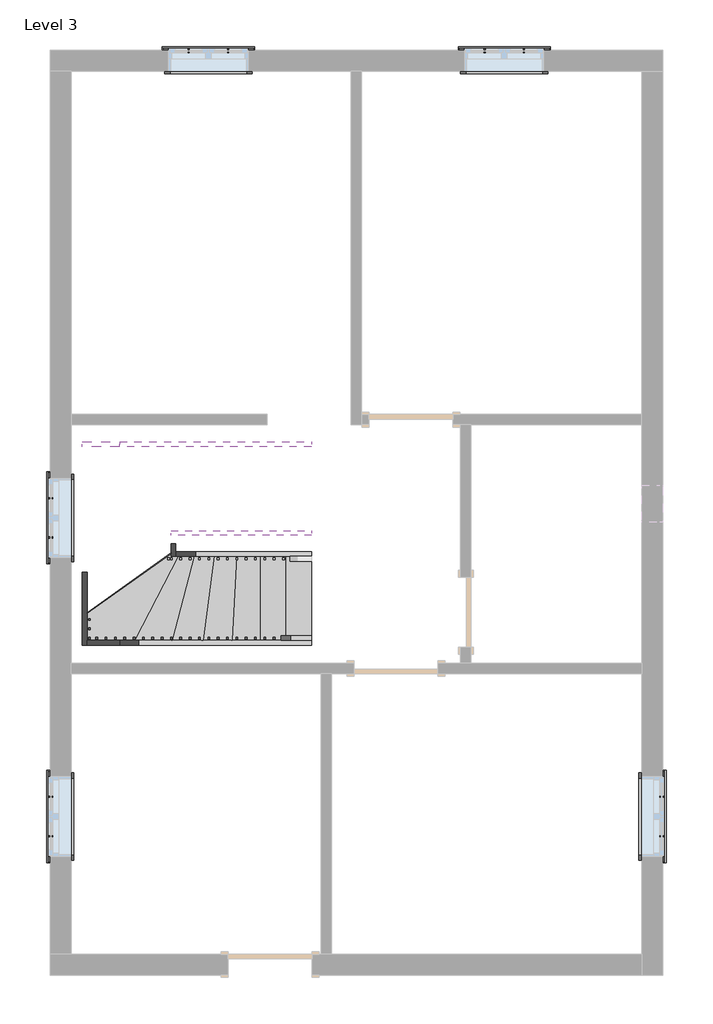
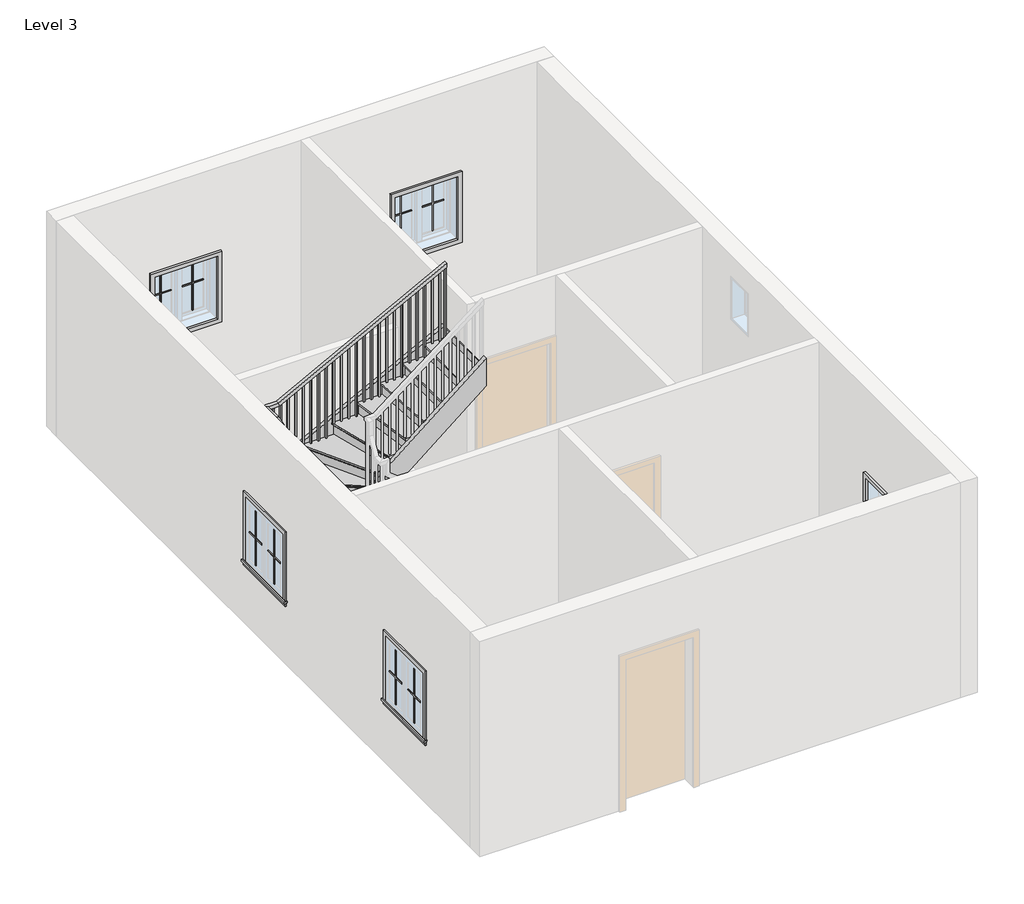
# One storey, part 2 of 2: 20 proxies, 8 members, 1 railing, 1 stair flight.
"""IFC4 building model written with IfcOpenShell, lengths in millimetres."""

from ifc_helpers import new_model, si_unit, frame, origin, place, context, project, spatial, polyline, outline, extrude, faceted_brep, transform, mapped, element, save
from components import muntin_pattern_2x2_muntin_pattern_2x2_b3fe6957, muntin_pattern_2x2_muntin_pattern_2x2_3e0ecaf2, trim_window_exterior_flat_with_sill_41619996, trim_window_interior_flat_picture_frame_51c85655, stair_flight_5420025d

model = new_model("IFC4")

# Units and contexts
model_context = context("Model", 3, world=origin())
ifc_project = project(units=[si_unit("LENGTHUNIT", "METRE", prefix="MILLI")], contexts=[model_context])

# Site, building, storey
site = spatial("IfcSite", under=ifc_project)
building = spatial("IfcBuilding", under=site)
storey = spatial("IfcBuildingStorey", under=building, Name="Level 3", Elevation=3200.4)

# Proxies
placement = place(None, origin())
muntin_pattern_2x2_muntin_pattern_2x2_shape = muntin_pattern_2x2_muntin_pattern_2x2_b3fe6957(model_context)
element("IfcBuildingElementProxy", 1, Name="Muntin Pattern_2x2 : Muntin Pattern_2x2", ObjectType="Muntin Pattern_2x2 : Muntin Pattern_2x2", at=placement, inside=storey, context=model_context, shape_type="MappedRepresentation", body=[
    mapped(muntin_pattern_2x2_muntin_pattern_2x2_shape, transform((-3096.8324167, 5150.2179147, 4184.65), x_axis=(1.0, 0.0, 0.0), y_axis=(0.0, 1.0, 0.0), z_axis=(0.0, 0.0, 1.0))),
])
element("IfcBuildingElementProxy", 2, Name="Muntin Pattern_2x2 : Muntin Pattern_2x2", ObjectType="Muntin Pattern_2x2 : Muntin Pattern_2x2", at=placement, inside=storey, context=model_context, shape_type="MappedRepresentation", body=[
    mapped(muntin_pattern_2x2_muntin_pattern_2x2_shape, transform((122.6175833, 5150.2179147, 4184.65), x_axis=(1.0, 0.0, 0.0), y_axis=(0.0, 1.0, 0.0), z_axis=(0.0, 0.0, 1.0))),
])
element("IfcBuildingElementProxy", 3, Name="Muntin Pattern_2x2 : Muntin Pattern_2x2", ObjectType="Muntin Pattern_2x2 : Muntin Pattern_2x2", at=placement, inside=storey, context=model_context, shape_type="MappedRepresentation", body=[
    mapped(muntin_pattern_2x2_muntin_pattern_2x2_shape, transform((-4597.0199167, -3388.9445853, 4184.65), x_axis=(0.0, 1.0, 0.0), y_axis=(-1.0, 0.0, 0.0), z_axis=(0.0, 0.0, 1.0))),
])
element("IfcBuildingElementProxy", 4, Name="Muntin Pattern_2x2 : Muntin Pattern_2x2", ObjectType="Muntin Pattern_2x2 : Muntin Pattern_2x2", at=placement, inside=storey, context=model_context, shape_type="MappedRepresentation", body=[
    mapped(muntin_pattern_2x2_muntin_pattern_2x2_shape, transform((2051.4300833, -2960.3195853, 4184.65), x_axis=(0.0, -1.0, 0.0), y_axis=(1.0, 0.0, 0.0), z_axis=(0.0, 0.0, 1.0))),
])
element("IfcBuildingElementProxy", 5, Name="Muntin Pattern_2x2 : Muntin Pattern_2x2", ObjectType="Muntin Pattern_2x2 : Muntin Pattern_2x2", at=placement, inside=storey, context=model_context, shape_type="MappedRepresentation", body=[
    mapped(muntin_pattern_2x2_muntin_pattern_2x2_shape, transform((-4597.0199167, -140.9195853, 4184.65), x_axis=(0.0, 1.0, 0.0), y_axis=(-1.0, 0.0, 0.0), z_axis=(0.0, 0.0, 1.0))),
])
muntin_pattern_2x2_muntin_pattern_2x2_2_shape = muntin_pattern_2x2_muntin_pattern_2x2_3e0ecaf2(model_context)
element("IfcBuildingElementProxy", 6, Name="Muntin Pattern_2x2 : Muntin Pattern_2x2", ObjectType="Muntin Pattern_2x2 : Muntin Pattern_2x2", at=placement, inside=storey, context=model_context, shape_type="MappedRepresentation", body=[
    mapped(muntin_pattern_2x2_muntin_pattern_2x2_2_shape, transform((-2668.2074167, 5150.2179147, 4184.65), x_axis=(-1.0, 0.0, 0.0), y_axis=(0.0, -1.0, 0.0), z_axis=(0.0, 0.0, 1.0))),
])
element("IfcBuildingElementProxy", 7, Name="Muntin Pattern_2x2 : Muntin Pattern_2x2", ObjectType="Muntin Pattern_2x2 : Muntin Pattern_2x2", at=placement, inside=storey, context=model_context, shape_type="MappedRepresentation", body=[
    mapped(muntin_pattern_2x2_muntin_pattern_2x2_2_shape, transform((551.2425833, 5150.2179147, 4184.65), x_axis=(-1.0, 0.0, 0.0), y_axis=(0.0, -1.0, 0.0), z_axis=(0.0, 0.0, 1.0))),
])
element("IfcBuildingElementProxy", 8, Name="Muntin Pattern_2x2 : Muntin Pattern_2x2", ObjectType="Muntin Pattern_2x2 : Muntin Pattern_2x2", at=placement, inside=storey, context=model_context, shape_type="MappedRepresentation", body=[
    mapped(muntin_pattern_2x2_muntin_pattern_2x2_2_shape, transform((-4597.0199167, -2960.3195853, 4184.65), x_axis=(0.0, -1.0, 0.0), y_axis=(1.0, 0.0, 0.0), z_axis=(0.0, 0.0, 1.0))),
])
element("IfcBuildingElementProxy", 9, Name="Muntin Pattern_2x2 : Muntin Pattern_2x2", ObjectType="Muntin Pattern_2x2 : Muntin Pattern_2x2", at=placement, inside=storey, context=model_context, shape_type="MappedRepresentation", body=[
    mapped(muntin_pattern_2x2_muntin_pattern_2x2_2_shape, transform((2051.4300833, -3388.9445853, 4184.65), x_axis=(0.0, 1.0, 0.0), y_axis=(-1.0, 0.0, 0.0), z_axis=(0.0, 0.0, 1.0))),
])
element("IfcBuildingElementProxy", 10, Name="Muntin Pattern_2x2 : Muntin Pattern_2x2", ObjectType="Muntin Pattern_2x2 : Muntin Pattern_2x2", at=placement, inside=storey, context=model_context, shape_type="MappedRepresentation", body=[
    mapped(muntin_pattern_2x2_muntin_pattern_2x2_2_shape, transform((-4597.0199167, 287.7054147, 4184.65), x_axis=(0.0, -1.0, 0.0), y_axis=(1.0, 0.0, 0.0), z_axis=(0.0, 0.0, 1.0))),
])
trim_window_exterior_flat_with_sill_shape = trim_window_exterior_flat_with_sill_41619996(model_context)
element("IfcBuildingElementProxy", 11, Name="Trim-Window-Exterior-Flat : with Sill", ObjectType="Trim-Window-Exterior-Flat : with Sill", at=placement, inside=storey, context=model_context, shape_type="MappedRepresentation", body=[
    mapped(trim_window_exterior_flat_with_sill_shape, transform((-2882.5199167, 5159.7429147, 5029.2), x_axis=(-1.0, 0.0, 0.0), y_axis=(0.0, 0.0, 1.0), z_axis=(0.0, 1.0, 0.0))),
])
element("IfcBuildingElementProxy", 12, Name="Trim-Window-Exterior-Flat : with Sill", ObjectType="Trim-Window-Exterior-Flat : with Sill", at=placement, inside=storey, context=model_context, shape_type="MappedRepresentation", body=[
    mapped(trim_window_exterior_flat_with_sill_shape, transform((336.9300833, 5159.7429147, 5029.2), x_axis=(-1.0, 0.0, 0.0), y_axis=(0.0, 0.0, 1.0), z_axis=(0.0, 1.0, 0.0))),
])
element("IfcBuildingElementProxy", 13, Name="Trim-Window-Exterior-Flat : with Sill", ObjectType="Trim-Window-Exterior-Flat : with Sill", at=placement, inside=storey, context=model_context, shape_type="MappedRepresentation", body=[
    mapped(trim_window_exterior_flat_with_sill_shape, transform((-4606.5449167, -3174.6320853, 5029.2), x_axis=(0.0, -1.0, 0.0), y_axis=(0.0, 0.0, 1.0), z_axis=(-1.0, 0.0, 0.0))),
])
element("IfcBuildingElementProxy", 14, Name="Trim-Window-Exterior-Flat : with Sill", ObjectType="Trim-Window-Exterior-Flat : with Sill", at=placement, inside=storey, context=model_context, shape_type="MappedRepresentation", body=[
    mapped(trim_window_exterior_flat_with_sill_shape, transform((2060.9550833, -3174.6320853, 5029.2), x_axis=(0.0, 1.0, 0.0), y_axis=(0.0, 0.0, 1.0), z_axis=(1.0, 0.0, 0.0))),
])
element("IfcBuildingElementProxy", 15, Name="Trim-Window-Exterior-Flat : with Sill", ObjectType="Trim-Window-Exterior-Flat : with Sill", at=placement, inside=storey, context=model_context, shape_type="MappedRepresentation", body=[
    mapped(trim_window_exterior_flat_with_sill_shape, transform((-4606.5449167, 73.3929147, 5029.2), x_axis=(0.0, -1.0, 0.0), y_axis=(0.0, 0.0, 1.0), z_axis=(-1.0, 0.0, 0.0))),
])
trim_window_interior_flat_picture_frame_shape = trim_window_interior_flat_picture_frame_51c85655(model_context)
element("IfcBuildingElementProxy", 16, Name="Trim-Window-Interior-Flat : Picture Frame", ObjectType="Trim-Window-Interior-Flat : Picture Frame", at=placement, inside=storey, context=model_context, shape_type="MappedRepresentation", body=[
    mapped(trim_window_interior_flat_picture_frame_shape, transform((-2882.5199167, 4931.1429147, 5029.2), x_axis=(1.0, 0.0, 0.0), y_axis=(0.0, 0.0, 1.0), z_axis=(0.0, -1.0, 0.0))),
])
element("IfcBuildingElementProxy", 17, Name="Trim-Window-Interior-Flat : Picture Frame", ObjectType="Trim-Window-Interior-Flat : Picture Frame", at=placement, inside=storey, context=model_context, shape_type="MappedRepresentation", body=[
    mapped(trim_window_interior_flat_picture_frame_shape, transform((336.9300833, 4931.1429147, 5029.2), x_axis=(1.0, 0.0, 0.0), y_axis=(0.0, 0.0, 1.0), z_axis=(0.0, -1.0, 0.0))),
])
element("IfcBuildingElementProxy", 18, Name="Trim-Window-Interior-Flat : Picture Frame", ObjectType="Trim-Window-Interior-Flat : Picture Frame", at=placement, inside=storey, context=model_context, shape_type="MappedRepresentation", body=[
    mapped(trim_window_interior_flat_picture_frame_shape, transform((-4377.9449167, -3174.6320853, 5029.2), x_axis=(0.0, 1.0, 0.0), y_axis=(0.0, 0.0, 1.0), z_axis=(1.0, 0.0, 0.0))),
])
element("IfcBuildingElementProxy", 19, Name="Trim-Window-Interior-Flat : Picture Frame", ObjectType="Trim-Window-Interior-Flat : Picture Frame", at=placement, inside=storey, context=model_context, shape_type="MappedRepresentation", body=[
    mapped(trim_window_interior_flat_picture_frame_shape, transform((1832.3550833, -3174.6320853, 5029.2), x_axis=(0.0, -1.0, 0.0), y_axis=(0.0, 0.0, 1.0), z_axis=(-1.0, 0.0, 0.0))),
])
element("IfcBuildingElementProxy", 20, Name="Trim-Window-Interior-Flat : Picture Frame", ObjectType="Trim-Window-Interior-Flat : Picture Frame", at=placement, inside=storey, context=model_context, shape_type="MappedRepresentation", body=[
    mapped(trim_window_interior_flat_picture_frame_shape, transform((-4377.9449167, 73.3929147, 5029.2), x_axis=(0.0, 1.0, 0.0), y_axis=(0.0, 0.0, 1.0), z_axis=(1.0, 0.0, 0.0))),
])

# Members
element("IfcMember", 21, ObjectType="Stringer - 2\" Width", at=placement, inside=storey, context=model_context, shape_type="SweptSolid", body=[
    extrude(outline(polyline([(3200.4, -1761.7449167), (3430.039954, -1761.7449167), (4505.7956453, -3849.1621084), (4162.900629, -3849.1621084), (3200.4, -1981.5072342), (3200.4, -1761.7449167)])), frame((0.0, -1310.9070853, 0.0), z_axis=(0.0, 1.0, 0.0), x_axis=(0.0, 0.0, 1.0)), (0.0, 0.0, 1.0), 50.8),
])
element("IfcMember", 22, ObjectType="Stringer - 2\" Width", at=placement, inside=storey, context=model_context, shape_type="SweptSolid", body=[
    extrude(outline(polyline([(-3849.1621084, -1260.1070853), (-3849.1621084, -1310.9070853), (-4203.8766085, -1310.9070853), (-4203.8766085, -1260.1070853), (-3849.1621084, -1260.1070853)])), frame((0.0, 0.0, 4162.900629), z_axis=(0.0, 0.0, 1.0), x_axis=(1.0, 0.0, 0.0)), (0.0, 0.0, 1.0), 342.8950162),
])
element("IfcMember", 23, ObjectType="Stringer - 2\" Width", at=placement, inside=storey, context=model_context, shape_type="SweptSolid", body=[
    extrude(outline(polyline([(-1310.9070853, 4200.9956453), (-1310.9070853, 4489.4952212), (811.1127974, 5170.3972697), (848.0929147, 5170.3972697), (848.0929147, 4839.3682298), (-1141.3846024, 4200.9956453), (-1310.9070853, 4200.9956453)])), frame((-4254.6766085, 0.0, 0.0), z_axis=(1.0, 0.0, 0.0), x_axis=(0.0, 1.0, 0.0)), (0.0, 0.0, 1.0), 50.8),
])
element("IfcMember", 24, ObjectType="Stringer - 2\" Width", at=placement, inside=storey, context=model_context, shape_type="SweptSolid", body=[
    extrude(outline(polyline([(-4254.6766085, 848.0929147), (-4254.6766085, 898.8929147), (-3849.1621084, 898.8929147), (-3849.1621084, 848.0929147), (-4254.6766085, 848.0929147)])), frame((0.0, 0.0, 4850.2904473), z_axis=(0.0, 0.0, 1.0), x_axis=(1.0, 0.0, 0.0)), (0.0, 0.0, 1.0), 320.1068224),
])
element("IfcMember", 25, ObjectType="Stringer - 2\" Width", at=placement, inside=storey, context=model_context, shape_type="SweptSolid", body=[
    extrude(outline(polyline([(5170.3972697, -3849.1621084), (4850.2904473, -3849.1621084), (5926.0461385, -1761.7449167), (6246.1529609, -1761.7449167), (5170.3972697, -3849.1621084)])), frame((0.0, 848.0929147, 0.0), z_axis=(0.0, 1.0, 0.0), x_axis=(0.0, 0.0, 1.0)), (0.0, 0.0, 1.0), 50.8),
])
element("IfcMember", 26, ObjectType="Stringer - 2\" Width", at=placement, inside=storey, context=model_context, shape_type="SweptSolid", body=[
    extrude(outline(polyline([(3200.4, -1761.7449167), (3376.5764461, -1761.7449167), (4580.818648, -3238.6766085), (4187.5410923, -3238.6766085), (3200.4, -2028.0065612), (3200.4, -1761.7449167)])), frame((0.0, -345.7070853, 0.0), z_axis=(0.0, 1.0, 0.0), x_axis=(0.0, 0.0, 1.0)), (0.0, 0.0, 1.0), 50.8),
])
element("IfcMember", 27, ObjectType="Stringer - 2\" Width", at=placement, inside=storey, context=model_context, shape_type="SweptSolid", body=[
    extrude(outline(polyline([(-345.7070853, 4228.9617647), (-345.7070853, 4773.6682978), (-139.0699679, 5126.5409689), (-117.1070853, 5126.5409689), (-117.1070853, 4560.865107), (-311.464868, 4228.9617647), (-345.7070853, 4228.9617647)])), frame((-3289.4766085, 0.0, 0.0), z_axis=(1.0, 0.0, 0.0), x_axis=(0.0, 1.0, 0.0)), (0.0, 0.0, 1.0), 50.8),
])
element("IfcMember", 28, ObjectType="Stringer - 2\" Width", at=placement, inside=storey, context=model_context, shape_type="SweptSolid", body=[
    extrude(outline(polyline([(5126.5409689, -3289.4766085), (4733.2634131, -3289.4766085), (5978.9262875, -1761.7449167), (6372.2038432, -1761.7449167), (5126.5409689, -3289.4766085)])), frame((0.0, -117.1070853, 0.0), z_axis=(0.0, 1.0, 0.0), x_axis=(0.0, 0.0, 1.0)), (0.0, 0.0, 1.0), 50.8),
])

# Railing
element("IfcRailing", 29, ObjectType="Handrail - Rectangular", at=placement, inside=storey, context=model_context, shape_type="SolidModel", body=[
    faceted_brep([(-1761.7449167, -1260.1070853, 4284.1333333), (-1761.7449167, -1260.1070853, 4226.6742652), (-1761.7449167, -1209.3070853, 4226.6742652), (-1761.7449167, -1209.3070853, 4284.1333333), (-4019.4699787, -1260.1070853, 5477.4239201), (-4032.0690433, -1260.1070853, 5426.6239201), (-4032.0690433, -1209.3070853, 5426.6239201), (-4019.4699787, -1209.3070853, 5477.4239201), (-4203.8766085, -1260.1070853, 5477.4239201), (-4203.8766085, -1260.1070853, 5426.6239201), (-4153.0766085, -1209.3070853, 5426.6239201), (-4153.0766085, -1209.3070853, 5477.4239201), (-4203.8766085, -972.7952032, 5477.4239201), (-4203.8766085, -964.8446271, 5426.6239201), (-4153.0766085, -964.8446271, 5426.6239201), (-4153.0766085, -972.7952032, 5477.4239201), (-4203.8766085, 560.7810325, 5969.5094132), (-4203.8766085, 568.7316087, 5918.7094132), (-4153.0766085, 568.7316087, 5918.7094132), (-4153.0766085, 560.7810325, 5969.5094132), (-4203.8766085, 848.0929147, 5969.5094132), (-4203.8766085, 848.0929147, 5918.7094132), (-4153.0766085, 797.2929147, 5918.7094132), (-4153.0766085, 797.2929147, 5969.5094132), (-4019.4699787, 848.0929147, 5969.5094132), (-4006.8709142, 848.0929147, 5918.7094132), (-4006.8709142, 797.2929147, 5918.7094132), (-4019.4699787, 797.2929147, 5969.5094132), (-1761.7449167, 848.0929147, 7162.8), (-1761.7449167, 797.2929147, 7162.8), (-1761.7449167, 797.2929147, 7105.3409318), (-1761.7449167, 848.0929147, 7105.3409318)], [[[0, 1, 2, 3]], [[1, 0, 4, 5]], [[2, 1, 5, 6]], [[3, 2, 6, 7]], [[0, 3, 7, 4]], [[5, 4, 8, 9]], [[6, 5, 9, 10]], [[7, 6, 10, 11]], [[4, 7, 11, 8]], [[9, 8, 12, 13]], [[10, 9, 13, 14]], [[11, 10, 14, 15]], [[8, 11, 15, 12]], [[13, 12, 16, 17]], [[14, 13, 17, 18]], [[15, 14, 18, 19]], [[12, 15, 19, 16]], [[17, 16, 20, 21]], [[18, 17, 21, 22]], [[19, 18, 22, 23]], [[16, 19, 23, 20]], [[21, 20, 24, 25]], [[22, 21, 25, 26]], [[23, 22, 26, 27]], [[20, 23, 27, 24]], [[28, 29, 30, 31]], [[25, 24, 28, 31]], [[26, 25, 31, 30]], [[27, 26, 30, 29]], [[24, 27, 29, 28]]]),
    extrude(outline(polyline([(7058.0597858, -1851.2016085), (6079.0666667, -1851.2016085), (6079.0666667, -1832.1516085), (7068.1284102, -1832.1516085), (7058.0597858, -1851.2016085)])), frame((0.0, 813.1679147, 0.0), z_axis=(0.0, 1.0, 0.0), x_axis=(0.0, 0.0, 1.0)), (0.0, 0.0, 1.0), 19.05),
    extrude(outline(polyline([(7004.3604556, -1952.8016085), (6079.0666667, -1952.8016085), (6079.0666667, -1933.7516085), (7014.42908, -1933.7516085), (7004.3604556, -1952.8016085)])), frame((0.0, 813.1679147, 0.0), z_axis=(0.0, 1.0, 0.0), x_axis=(0.0, 0.0, 1.0)), (0.0, 0.0, 1.0), 19.05),
    extrude(outline(polyline([(6950.6611254, -2054.4016085), (5909.7333333, -2054.4016085), (5909.7333333, -2035.3516085), (6960.7297498, -2035.3516085), (6950.6611254, -2054.4016085)])), frame((0.0, 813.1679147, 0.0), z_axis=(0.0, 1.0, 0.0), x_axis=(0.0, 0.0, 1.0)), (0.0, 0.0, 1.0), 19.05),
    extrude(outline(polyline([(6896.9617952, -2156.0016085), (5909.7333333, -2156.0016085), (5909.7333333, -2136.9516085), (6907.0304196, -2136.9516085), (6896.9617952, -2156.0016085)])), frame((0.0, 813.1679147, 0.0), z_axis=(0.0, 1.0, 0.0), x_axis=(0.0, 0.0, 1.0)), (0.0, 0.0, 1.0), 19.05),
    extrude(outline(polyline([(6843.262465, -2257.6016085), (5909.7333333, -2257.6016085), (5909.7333333, -2238.5516085), (6853.3310894, -2238.5516085), (6843.262465, -2257.6016085)])), frame((0.0, 813.1679147, 0.0), z_axis=(0.0, 1.0, 0.0), x_axis=(0.0, 0.0, 1.0)), (0.0, 0.0, 1.0), 19.05),
    extrude(outline(polyline([(6789.5631348, -2359.2016085), (5740.4, -2359.2016085), (5740.4, -2340.1516085), (6799.6317592, -2340.1516085), (6789.5631348, -2359.2016085)])), frame((0.0, 813.1679147, 0.0), z_axis=(0.0, 1.0, 0.0), x_axis=(0.0, 0.0, 1.0)), (0.0, 0.0, 1.0), 19.05),
    extrude(outline(polyline([(6735.8638046, -2460.8016085), (5740.4, -2460.8016085), (5740.4, -2441.7516085), (6745.932429, -2441.7516085), (6735.8638046, -2460.8016085)])), frame((0.0, 813.1679147, 0.0), z_axis=(0.0, 1.0, 0.0), x_axis=(0.0, 0.0, 1.0)), (0.0, 0.0, 1.0), 19.05),
    extrude(outline(polyline([(6682.1644744, -2562.4016085), (5740.4, -2562.4016085), (5740.4, -2543.3516085), (6692.2330988, -2543.3516085), (6682.1644744, -2562.4016085)])), frame((0.0, 813.1679147, 0.0), z_axis=(0.0, 1.0, 0.0), x_axis=(0.0, 0.0, 1.0)), (0.0, 0.0, 1.0), 19.05),
    extrude(outline(polyline([(6628.4651442, -2664.0016085), (5571.0666667, -2664.0016085), (5571.0666667, -2644.9516085), (6638.5337686, -2644.9516085), (6628.4651442, -2664.0016085)])), frame((0.0, 813.1679147, 0.0), z_axis=(0.0, 1.0, 0.0), x_axis=(0.0, 0.0, 1.0)), (0.0, 0.0, 1.0), 19.05),
    extrude(outline(polyline([(6574.765814, -2765.6016085), (5571.0666667, -2765.6016085), (5571.0666667, -2746.5516085), (6584.8344384, -2746.5516085), (6574.765814, -2765.6016085)])), frame((0.0, 813.1679147, 0.0), z_axis=(0.0, 1.0, 0.0), x_axis=(0.0, 0.0, 1.0)), (0.0, 0.0, 1.0), 19.05),
    extrude(outline(polyline([(6521.0664838, -2867.2016085), (5571.0666667, -2867.2016085), (5571.0666667, -2848.1516085), (6531.1351082, -2848.1516085), (6521.0664838, -2867.2016085)])), frame((0.0, 813.1679147, 0.0), z_axis=(0.0, 1.0, 0.0), x_axis=(0.0, 0.0, 1.0)), (0.0, 0.0, 1.0), 19.05),
    extrude(outline(polyline([(6467.3671536, -2968.8016085), (5401.7333333, -2968.8016085), (5401.7333333, -2949.7516085), (6477.435778, -2949.7516085), (6467.3671536, -2968.8016085)])), frame((0.0, 813.1679147, 0.0), z_axis=(0.0, 1.0, 0.0), x_axis=(0.0, 0.0, 1.0)), (0.0, 0.0, 1.0), 19.05),
    extrude(outline(polyline([(6413.6678234, -3070.4016085), (5401.7333333, -3070.4016085), (5401.7333333, -3051.3516085), (6423.7364478, -3051.3516085), (6413.6678234, -3070.4016085)])), frame((0.0, 813.1679147, 0.0), z_axis=(0.0, 1.0, 0.0), x_axis=(0.0, 0.0, 1.0)), (0.0, 0.0, 1.0), 19.05),
    extrude(outline(polyline([(6359.9684932, -3172.0016085), (5401.7333333, -3172.0016085), (5401.7333333, -3152.9516085), (6370.0371176, -3152.9516085), (6359.9684932, -3172.0016085)])), frame((0.0, 813.1679147, 0.0), z_axis=(0.0, 1.0, 0.0), x_axis=(0.0, 0.0, 1.0)), (0.0, 0.0, 1.0), 19.05),
    extrude(outline(polyline([(6306.269163, -3273.6016085), (5401.7333333, -3273.6016085), (5401.7333333, -3254.5516085), (6316.3377874, -3254.5516085), (6306.269163, -3273.6016085)])), frame((0.0, 813.1679147, 0.0), z_axis=(0.0, 1.0, 0.0), x_axis=(0.0, 0.0, 1.0)), (0.0, 0.0, 1.0), 19.05),
    extrude(outline(polyline([(6252.5698328, -3375.2016085), (5232.4, -3375.2016085), (5232.4, -3356.1516085), (6262.6384572, -3356.1516085), (6252.5698328, -3375.2016085)])), frame((0.0, 813.1679147, 0.0), z_axis=(0.0, 1.0, 0.0), x_axis=(0.0, 0.0, 1.0)), (0.0, 0.0, 1.0), 19.05),
    extrude(outline(polyline([(6198.8705026, -3476.8016085), (5232.4, -3476.8016085), (5232.4, -3457.7516085), (6208.939127, -3457.7516085), (6198.8705026, -3476.8016085)])), frame((0.0, 813.1679147, 0.0), z_axis=(0.0, 1.0, 0.0), x_axis=(0.0, 0.0, 1.0)), (0.0, 0.0, 1.0), 19.05),
    extrude(outline(polyline([(6145.1711724, -3578.4016085), (5232.4, -3578.4016085), (5232.4, -3559.3516085), (6155.2397968, -3559.3516085), (6145.1711724, -3578.4016085)])), frame((0.0, 813.1679147, 0.0), z_axis=(0.0, 1.0, 0.0), x_axis=(0.0, 0.0, 1.0)), (0.0, 0.0, 1.0), 19.05),
    extrude(outline(polyline([(6091.4718422, -3680.0016085), (5232.4, -3680.0016085), (5232.4, -3660.9516085), (6101.5404666, -3660.9516085), (6091.4718422, -3680.0016085)])), frame((0.0, 813.1679147, 0.0), z_axis=(0.0, 1.0, 0.0), x_axis=(0.0, 0.0, 1.0)), (0.0, 0.0, 1.0), 19.05),
    extrude(outline(polyline([(6037.772512, -3781.6016085), (5063.0666667, -3781.6016085), (5063.0666667, -3762.5516085), (6047.8411364, -3762.5516085), (6037.772512, -3781.6016085)])), frame((0.0, 813.1679147, 0.0), z_axis=(0.0, 1.0, 0.0), x_axis=(0.0, 0.0, 1.0)), (0.0, 0.0, 1.0), 19.05),
    extrude(outline(polyline([(5984.0731818, -3883.2016085), (5063.0666667, -3883.2016085), (5063.0666667, -3864.1516085), (5994.1418062, -3864.1516085), (5984.0731818, -3883.2016085)])), frame((0.0, 813.1679147, 0.0), z_axis=(0.0, 1.0, 0.0), x_axis=(0.0, 0.0, 1.0)), (0.0, 0.0, 1.0), 19.05),
    extrude(outline(polyline([(5930.3738516, -3984.8016085), (5063.0666667, -3984.8016085), (5063.0666667, -3965.7516085), (5940.442476, -3965.7516085), (5930.3738516, -3984.8016085)])), frame((0.0, 813.1679147, 0.0), z_axis=(0.0, 1.0, 0.0), x_axis=(0.0, 0.0, 1.0)), (0.0, 0.0, 1.0), 19.05),
    extrude(outline(polyline([(-4086.4016085, 832.2179147), (-4067.3516085, 832.2179147), (-4067.3516085, 813.1679147), (-4086.4016085, 813.1679147), (-4086.4016085, 832.2179147)])), frame((0.0, 0.0, 5063.0666667), z_axis=(0.0, 0.0, 1.0), x_axis=(1.0, 0.0, 0.0)), (0.0, 0.0, 1.0), 855.6427466),
    extrude(outline(polyline([(-4188.0016085, 787.7679147), (-4188.0016085, 806.8179147), (-4168.9516085, 806.8179147), (-4168.9516085, 787.7679147), (-4188.0016085, 787.7679147)])), frame((0.0, 0.0, 5063.0666667), z_axis=(0.0, 0.0, 1.0), x_axis=(1.0, 0.0, 0.0)), (0.0, 0.0, 1.0), 855.6427466),
    extrude(outline(polyline([(-4188.0016085, 686.1679147), (-4188.0016085, 705.2179147), (-4168.9516085, 705.2179147), (-4168.9516085, 686.1679147), (-4188.0016085, 686.1679147)])), frame((0.0, 0.0, 5063.0666667), z_axis=(0.0, 0.0, 1.0), x_axis=(1.0, 0.0, 0.0)), (0.0, 0.0, 1.0), 855.6427466),
    extrude(outline(polyline([(-4188.0016085, 584.5679147), (-4188.0016085, 603.6179147), (-4168.9516085, 603.6179147), (-4168.9516085, 584.5679147), (-4188.0016085, 584.5679147)])), frame((0.0, 0.0, 5063.0666667), z_axis=(0.0, 0.0, 1.0), x_axis=(1.0, 0.0, 0.0)), (0.0, 0.0, 1.0), 855.6427466),
    extrude(outline(polyline([(502.0179147, 5897.3026907), (502.0179147, 4893.7333333), (482.9679147, 4893.7333333), (482.9679147, 5891.1900316), (502.0179147, 5897.3026907)])), frame((-4188.0016085, 0.0, 0.0), z_axis=(1.0, 0.0, 0.0), x_axis=(0.0, 1.0, 0.0)), (0.0, 0.0, 1.0), 19.05),
    extrude(outline(polyline([(400.4179147, 5864.7018425), (400.4179147, 4893.7333333), (381.3679147, 4893.7333333), (381.3679147, 5858.5891834), (400.4179147, 5864.7018425)])), frame((-4188.0016085, 0.0, 0.0), z_axis=(1.0, 0.0, 0.0), x_axis=(0.0, 1.0, 0.0)), (0.0, 0.0, 1.0), 19.05),
    extrude(outline(polyline([(298.8179147, 5832.1009942), (298.8179147, 4893.7333333), (279.7679147, 4893.7333333), (279.7679147, 5825.9883352), (298.8179147, 5832.1009942)])), frame((-4188.0016085, 0.0, 0.0), z_axis=(1.0, 0.0, 0.0), x_axis=(0.0, 1.0, 0.0)), (0.0, 0.0, 1.0), 19.05),
    extrude(outline(polyline([(197.2179147, 5799.500146), (197.2179147, 4893.7333333), (178.1679147, 4893.7333333), (178.1679147, 5793.387487), (197.2179147, 5799.500146)])), frame((-4188.0016085, 0.0, 0.0), z_axis=(1.0, 0.0, 0.0), x_axis=(0.0, 1.0, 0.0)), (0.0, 0.0, 1.0), 19.05),
    extrude(outline(polyline([(95.6179147, 5766.8992978), (95.6179147, 4893.7333333), (76.5679147, 4893.7333333), (76.5679147, 5760.7866387), (95.6179147, 5766.8992978)])), frame((-4188.0016085, 0.0, 0.0), z_axis=(1.0, 0.0, 0.0), x_axis=(0.0, 1.0, 0.0)), (0.0, 0.0, 1.0), 19.05),
    extrude(outline(polyline([(-5.9820853, 5734.2984495), (-5.9820853, 4724.4), (-25.0320853, 4724.4), (-25.0320853, 5728.1857905), (-5.9820853, 5734.2984495)])), frame((-4188.0016085, 0.0, 0.0), z_axis=(1.0, 0.0, 0.0), x_axis=(0.0, 1.0, 0.0)), (0.0, 0.0, 1.0), 19.05),
    extrude(outline(polyline([(-107.5820853, 5701.6976013), (-107.5820853, 4724.4), (-126.6320853, 4724.4), (-126.6320853, 5695.5849423), (-107.5820853, 5701.6976013)])), frame((-4188.0016085, 0.0, 0.0), z_axis=(1.0, 0.0, 0.0), x_axis=(0.0, 1.0, 0.0)), (0.0, 0.0, 1.0), 19.05),
    extrude(outline(polyline([(-209.1820853, 5669.0967531), (-209.1820853, 4724.4), (-228.2320853, 4724.4), (-228.2320853, 5662.9840941), (-209.1820853, 5669.0967531)])), frame((-4188.0016085, 0.0, 0.0), z_axis=(1.0, 0.0, 0.0), x_axis=(0.0, 1.0, 0.0)), (0.0, 0.0, 1.0), 19.05),
    extrude(outline(polyline([(-310.7820853, 5636.4959049), (-310.7820853, 4724.4), (-329.8320853, 4724.4), (-329.8320853, 5630.3832458), (-310.7820853, 5636.4959049)])), frame((-4188.0016085, 0.0, 0.0), z_axis=(1.0, 0.0, 0.0), x_axis=(0.0, 1.0, 0.0)), (0.0, 0.0, 1.0), 19.05),
    extrude(outline(polyline([(-412.3820853, 5603.8950566), (-412.3820853, 4724.4), (-431.4320853, 4724.4), (-431.4320853, 5597.7823976), (-412.3820853, 5603.8950566)])), frame((-4188.0016085, 0.0, 0.0), z_axis=(1.0, 0.0, 0.0), x_axis=(0.0, 1.0, 0.0)), (0.0, 0.0, 1.0), 19.05),
    extrude(outline(polyline([(-513.9820853, 5571.2942084), (-513.9820853, 4555.0666667), (-533.0320853, 4555.0666667), (-533.0320853, 5565.1815494), (-513.9820853, 5571.2942084)])), frame((-4188.0016085, 0.0, 0.0), z_axis=(1.0, 0.0, 0.0), x_axis=(0.0, 1.0, 0.0)), (0.0, 0.0, 1.0), 19.05),
    extrude(outline(polyline([(-615.5820853, 5538.6933602), (-615.5820853, 4555.0666667), (-634.6320853, 4555.0666667), (-634.6320853, 5532.5807011), (-615.5820853, 5538.6933602)])), frame((-4188.0016085, 0.0, 0.0), z_axis=(1.0, 0.0, 0.0), x_axis=(0.0, 1.0, 0.0)), (0.0, 0.0, 1.0), 19.05),
    extrude(outline(polyline([(-717.1820853, 5506.092512), (-717.1820853, 4555.0666667), (-736.2320853, 4555.0666667), (-736.2320853, 5499.9798529), (-717.1820853, 5506.092512)])), frame((-4188.0016085, 0.0, 0.0), z_axis=(1.0, 0.0, 0.0), x_axis=(0.0, 1.0, 0.0)), (0.0, 0.0, 1.0), 19.05),
    extrude(outline(polyline([(-818.7820853, 5473.4916637), (-818.7820853, 4555.0666667), (-837.8320853, 4555.0666667), (-837.8320853, 5467.3790047), (-818.7820853, 5473.4916637)])), frame((-4188.0016085, 0.0, 0.0), z_axis=(1.0, 0.0, 0.0), x_axis=(0.0, 1.0, 0.0)), (0.0, 0.0, 1.0), 19.05),
    extrude(outline(polyline([(-920.3820853, 5440.8908155), (-920.3820853, 4555.0666667), (-939.4320853, 4555.0666667), (-939.4320853, 5434.7781565), (-920.3820853, 5440.8908155)])), frame((-4188.0016085, 0.0, 0.0), z_axis=(1.0, 0.0, 0.0), x_axis=(0.0, 1.0, 0.0)), (0.0, 0.0, 1.0), 19.05),
    extrude(outline(polyline([(-4188.0016085, -1041.0320853), (-4188.0016085, -1021.9820853), (-4168.9516085, -1021.9820853), (-4168.9516085, -1041.0320853), (-4188.0016085, -1041.0320853)])), frame((0.0, 0.0, 4385.7333333), z_axis=(0.0, 0.0, 1.0), x_axis=(1.0, 0.0, 0.0)), (0.0, 0.0, 1.0), 1040.8905868),
    extrude(outline(polyline([(-4188.0016085, -1142.6320853), (-4188.0016085, -1123.5820853), (-4168.9516085, -1123.5820853), (-4168.9516085, -1142.6320853), (-4188.0016085, -1142.6320853)])), frame((0.0, 0.0, 4385.7333333), z_axis=(0.0, 0.0, 1.0), x_axis=(1.0, 0.0, 0.0)), (0.0, 0.0, 1.0), 1040.8905868),
    extrude(outline(polyline([(-4089.0199167, -1244.2320853), (-4108.0699167, -1244.2320853), (-4108.0699167, -1225.1820853), (-4089.0199167, -1225.1820853), (-4089.0199167, -1244.2320853)])), frame((0.0, 0.0, 4385.7333333), z_axis=(0.0, 0.0, 1.0), x_axis=(1.0, 0.0, 0.0)), (0.0, 0.0, 1.0), 1040.8905868),
    extrude(outline(polyline([(5413.0938418, -4006.4699167), (4385.7333333, -4006.4699167), (4385.7333333, -3987.4199167), (5403.0252174, -3987.4199167), (5413.0938418, -4006.4699167)])), frame((0.0, -1244.2320853, 0.0), z_axis=(0.0, 1.0, 0.0), x_axis=(0.0, 0.0, 1.0)), (0.0, 0.0, 1.0), 19.05),
    extrude(outline(polyline([(5359.3945116, -3904.8699167), (4385.7333333, -3904.8699167), (4385.7333333, -3885.8199167), (5349.3258872, -3885.8199167), (5359.3945116, -3904.8699167)])), frame((0.0, -1244.2320853, 0.0), z_axis=(0.0, 1.0, 0.0), x_axis=(0.0, 0.0, 1.0)), (0.0, 0.0, 1.0), 19.05),
    extrude(outline(polyline([(5305.6951814, -3803.2699167), (4385.7333333, -3803.2699167), (4385.7333333, -3784.2199167), (5295.626557, -3784.2199167), (5305.6951814, -3803.2699167)])), frame((0.0, -1244.2320853, 0.0), z_axis=(0.0, 1.0, 0.0), x_axis=(0.0, 0.0, 1.0)), (0.0, 0.0, 1.0), 19.05),
    extrude(outline(polyline([(5251.9958512, -3701.6699167), (4385.7333333, -3701.6699167), (4385.7333333, -3682.6199167), (5241.9272268, -3682.6199167), (5251.9958512, -3701.6699167)])), frame((0.0, -1244.2320853, 0.0), z_axis=(0.0, 1.0, 0.0), x_axis=(0.0, 0.0, 1.0)), (0.0, 0.0, 1.0), 19.05),
    extrude(outline(polyline([(5198.296521, -3600.0699167), (4216.4, -3600.0699167), (4216.4, -3581.0199167), (5188.2278966, -3581.0199167), (5198.296521, -3600.0699167)])), frame((0.0, -1244.2320853, 0.0), z_axis=(0.0, 1.0, 0.0), x_axis=(0.0, 0.0, 1.0)), (0.0, 0.0, 1.0), 19.05),
    extrude(outline(polyline([(5144.5971908, -3498.4699167), (4216.4, -3498.4699167), (4216.4, -3479.4199167), (5134.5285664, -3479.4199167), (5144.5971908, -3498.4699167)])), frame((0.0, -1244.2320853, 0.0), z_axis=(0.0, 1.0, 0.0), x_axis=(0.0, 0.0, 1.0)), (0.0, 0.0, 1.0), 19.05),
    extrude(outline(polyline([(5090.8978606, -3396.8699167), (4216.4, -3396.8699167), (4216.4, -3377.8199167), (5080.8292362, -3377.8199167), (5090.8978606, -3396.8699167)])), frame((0.0, -1244.2320853, 0.0), z_axis=(0.0, 1.0, 0.0), x_axis=(0.0, 0.0, 1.0)), (0.0, 0.0, 1.0), 19.05),
    extrude(outline(polyline([(5037.1985304, -3295.2699167), (4216.4, -3295.2699167), (4216.4, -3276.2199167), (5027.129906, -3276.2199167), (5037.1985304, -3295.2699167)])), frame((0.0, -1244.2320853, 0.0), z_axis=(0.0, 1.0, 0.0), x_axis=(0.0, 0.0, 1.0)), (0.0, 0.0, 1.0), 19.05),
    extrude(outline(polyline([(4983.4992002, -3193.6699167), (4047.0666667, -3193.6699167), (4047.0666667, -3174.6199167), (4973.4305758, -3174.6199167), (4983.4992002, -3193.6699167)])), frame((0.0, -1244.2320853, 0.0), z_axis=(0.0, 1.0, 0.0), x_axis=(0.0, 0.0, 1.0)), (0.0, 0.0, 1.0), 19.05),
    extrude(outline(polyline([(4929.79987, -3092.0699167), (4047.0666667, -3092.0699167), (4047.0666667, -3073.0199167), (4919.7312456, -3073.0199167), (4929.79987, -3092.0699167)])), frame((0.0, -1244.2320853, 0.0), z_axis=(0.0, 1.0, 0.0), x_axis=(0.0, 0.0, 1.0)), (0.0, 0.0, 1.0), 19.05),
    extrude(outline(polyline([(4876.1005398, -2990.4699167), (4047.0666667, -2990.4699167), (4047.0666667, -2971.4199167), (4866.0319154, -2971.4199167), (4876.1005398, -2990.4699167)])), frame((0.0, -1244.2320853, 0.0), z_axis=(0.0, 1.0, 0.0), x_axis=(0.0, 0.0, 1.0)), (0.0, 0.0, 1.0), 19.05),
    extrude(outline(polyline([(4822.4012096, -2888.8699167), (3877.7333333, -2888.8699167), (3877.7333333, -2869.8199167), (4812.3325852, -2869.8199167), (4822.4012096, -2888.8699167)])), frame((0.0, -1244.2320853, 0.0), z_axis=(0.0, 1.0, 0.0), x_axis=(0.0, 0.0, 1.0)), (0.0, 0.0, 1.0), 19.05),
    extrude(outline(polyline([(4768.7018794, -2787.2699167), (3877.7333333, -2787.2699167), (3877.7333333, -2768.2199167), (4758.633255, -2768.2199167), (4768.7018794, -2787.2699167)])), frame((0.0, -1244.2320853, 0.0), z_axis=(0.0, 1.0, 0.0), x_axis=(0.0, 0.0, 1.0)), (0.0, 0.0, 1.0), 19.05),
    extrude(outline(polyline([(4715.0025492, -2685.6699167), (3877.7333333, -2685.6699167), (3877.7333333, -2666.6199167), (4704.9339248, -2666.6199167), (4715.0025492, -2685.6699167)])), frame((0.0, -1244.2320853, 0.0), z_axis=(0.0, 1.0, 0.0), x_axis=(0.0, 0.0, 1.0)), (0.0, 0.0, 1.0), 19.05),
    extrude(outline(polyline([(4661.303219, -2584.0699167), (3708.4, -2584.0699167), (3708.4, -2565.0199167), (4651.2345946, -2565.0199167), (4661.303219, -2584.0699167)])), frame((0.0, -1244.2320853, 0.0), z_axis=(0.0, 1.0, 0.0), x_axis=(0.0, 0.0, 1.0)), (0.0, 0.0, 1.0), 19.05),
    extrude(outline(polyline([(4607.6038888, -2482.4699167), (3708.4, -2482.4699167), (3708.4, -2463.4199167), (4597.5352644, -2463.4199167), (4607.6038888, -2482.4699167)])), frame((0.0, -1244.2320853, 0.0), z_axis=(0.0, 1.0, 0.0), x_axis=(0.0, 0.0, 1.0)), (0.0, 0.0, 1.0), 19.05),
    extrude(outline(polyline([(4553.9045586, -2380.8699167), (3708.4, -2380.8699167), (3708.4, -2361.8199167), (4543.8359342, -2361.8199167), (4553.9045586, -2380.8699167)])), frame((0.0, -1244.2320853, 0.0), z_axis=(0.0, 1.0, 0.0), x_axis=(0.0, 0.0, 1.0)), (0.0, 0.0, 1.0), 19.05),
    extrude(outline(polyline([(4500.2052284, -2279.2699167), (3539.0666667, -2279.2699167), (3539.0666667, -2260.2199167), (4490.136604, -2260.2199167), (4500.2052284, -2279.2699167)])), frame((0.0, -1244.2320853, 0.0), z_axis=(0.0, 1.0, 0.0), x_axis=(0.0, 0.0, 1.0)), (0.0, 0.0, 1.0), 19.05),
    extrude(outline(polyline([(4446.5058982, -2177.6699167), (3539.0666667, -2177.6699167), (3539.0666667, -2158.6199167), (4436.4372738, -2158.6199167), (4446.5058982, -2177.6699167)])), frame((0.0, -1244.2320853, 0.0), z_axis=(0.0, 1.0, 0.0), x_axis=(0.0, 0.0, 1.0)), (0.0, 0.0, 1.0), 19.05),
    extrude(outline(polyline([(4392.806568, -2076.0699167), (3539.0666667, -2076.0699167), (3539.0666667, -2057.0199167), (4382.7379436, -2057.0199167), (4392.806568, -2076.0699167)])), frame((0.0, -1244.2320853, 0.0), z_axis=(0.0, 1.0, 0.0), x_axis=(0.0, 0.0, 1.0)), (0.0, 0.0, 1.0), 19.05),
    extrude(outline(polyline([(4339.1072378, -1974.4699167), (3369.7333333, -1974.4699167), (3369.7333333, -1955.4199167), (4329.0386134, -1955.4199167), (4339.1072378, -1974.4699167)])), frame((0.0, -1244.2320853, 0.0), z_axis=(0.0, 1.0, 0.0), x_axis=(0.0, 0.0, 1.0)), (0.0, 0.0, 1.0), 19.05),
    extrude(outline(polyline([(4285.4079076, -1872.8699167), (3369.7333333, -1872.8699167), (3369.7333333, -1853.8199167), (4275.3392831, -1853.8199167), (4285.4079076, -1872.8699167)])), frame((0.0, -1244.2320853, 0.0), z_axis=(0.0, 1.0, 0.0), x_axis=(0.0, 0.0, 1.0)), (0.0, 0.0, 1.0), 19.05),
    extrude(outline(polyline([(-4188.0016085, 813.1679147), (-4188.0016085, 832.2179147), (-4168.9516085, 832.2179147), (-4168.9516085, 813.1679147), (-4188.0016085, 813.1679147)])), frame((0.0, 0.0, 5063.0666667), z_axis=(0.0, 0.0, 1.0), x_axis=(1.0, 0.0, 0.0)), (0.0, 0.0, 1.0), 855.6427466),
    extrude(outline(polyline([(-4168.9516085, -1244.2320853), (-4188.0016085, -1244.2320853), (-4188.0016085, -1225.1820853), (-4168.9516085, -1225.1820853), (-4168.9516085, -1244.2320853)])), frame((0.0, 0.0, 4385.7333333), z_axis=(0.0, 0.0, 1.0), x_axis=(1.0, 0.0, 0.0)), (0.0, 0.0, 1.0), 1040.8905868),
    extrude(outline(polyline([(7095.2723074, -1780.7949167), (6079.0666667, -1780.7949167), (6079.0666667, -1761.7449167), (7105.3409318, -1761.7449167), (7095.2723074, -1780.7949167)])), frame((0.0, 813.1679147, 0.0), z_axis=(0.0, 1.0, 0.0), x_axis=(0.0, 0.0, 1.0)), (0.0, 0.0, 1.0), 19.05),
    extrude(outline(polyline([(4236.7428896, -1780.7949167), (3369.7333333, -1780.7949167), (3369.7333333, -1761.7449167), (4226.6742652, -1761.7449167), (4236.7428896, -1780.7949167)])), frame((0.0, -1244.2320853, 0.0), z_axis=(0.0, 1.0, 0.0), x_axis=(0.0, 0.0, 1.0)), (0.0, 0.0, 1.0), 19.05),
])

# Stair flight
stair_flight_shape = stair_flight_5420025d(model_context)
element("IfcStairFlight", 30, ObjectType="2\" Tread 1\" Nosing 1/4\" Riser", at=placement, inside=storey, context=model_context, shape_type="MappedRepresentation", body=[
    mapped(stair_flight_shape, transform((0.0, 0.0, 0.0), x_axis=(1.0, 0.0, 0.0), y_axis=(0.0, 1.0, 0.0), z_axis=(0.0, 0.0, 1.0))),
])

save(model, "model.ifc")

# Revit data of these elements
# Type "Muntin Pattern_2x2 : Muntin Pattern_2x2"
#   Width [instance default] = 4' - 0"
#   Thickness = 0' - 0 1/2"
#   Height [instance default] = 4' - 0"
#   Distance = 0' - 0 3/4"
#   Interior Material [instance default] = none
#   Exterior Material [instance default] = none
#   Default Elevation = 0
# Type "Trim-Window-Exterior-Flat : with Sill"
#   Trim Width = 0' - 2 1/4"
#   Trim Thickness_Picture Frame = 0' - 1 1/4"
#   Trim Thickness_with Sill = 0' - 0 3/4"
#   Sill Thickness = 0' - 1 1/4"
#   Opening Width [instance default] = 2' - 0"
#   Opening Height [instance default] = 3' - 0"
#   Default Elevation = 4' - 0"
#   Sill = yes
#   Picture Frame = no
#   Trim Material [instance default] = none
# Type "Trim-Window-Interior-Flat : Picture Frame"
#   Trim Thickness_Picture Frame = 0' - 1 1/4"
#   Trim Width = 0' - 2 1/4"
#   Trim Thickness_with Sill = 0' - 0 3/4"
#   Sill Thickness = 0' - 1 1/4"
#   Opening Width [instance default] = 2' - 0"
#   Opening Height [instance default] = 3' - 0"
#   Default Elevation = 4' - 0"
#   Sill = no
#   Picture Frame = yes
#   Trim Material [instance default] = none
# Type "Handrail - Rectangular"
#   Assembly Code = "C2010400"
#   built-in parameter 1008612 = 0.0416667 (stored number, unit not read)
#   built-in parameter 1008611 = 0.0416667 (stored number, unit not read)
#   built-in parameter 1008609 = 0.333333 (stored number, unit not read)
#   built-in parameter 1008604 = 0.166667 (stored number, unit not read)
#   built-in parameter 1008603 = 0.166667 (stored number, unit not read)
#   Railing Height = 3' - 0"
#   built-in parameter 1008630 = 2
#   built-in parameter 1008610 = 2
#   built-in parameter 1008618 = Baluster - Square : 3/4"
# Elements 1, 2, 3, 4, 5, 6, 7, 8, 9, 10 (IfcBuildingElementProxy, "Muntin Pattern_2x2 : Muntin Pattern_2x2")
#   Width = 0' - 11 5/8"
#   Height = 2' - 6 1/2"
#   Interior Material = Wood - Stained
#   Exterior Material = Clad - White
#   Phase Created = New Construction
#   Materials on its faces: "Clad - White", "Wood - Stained"
# Elements 11, 12, 13, 14, 15 (IfcBuildingElementProxy, "Trim-Window-Exterior-Flat : with Sill")
#   Opening Width = 2' - 10"
#   Opening Height = 3' - 0"
#   Trim Material = Clad - White
#   Phase Created = New Construction
#   Materials on its faces: "Clad - White"
# Elements 16, 17, 18, 19, 20 (IfcBuildingElementProxy, "Trim-Window-Interior-Flat : Picture Frame")
#   Opening Width = 2' - 10"
#   Opening Height = 3' - 0"
#   Trim Material = Wood - Stained
#   Phase Created = New Construction
#   Materials on its faces: "Wood - Stained"
# Elements 21, 22, 23, 24, 25, 26, 27, 28 (IfcMember, "Stringer - 2\" Width")
#   Phase Created = New Construction
# Element 29 (IfcRailing, "Handrail - Rectangular")
#   Phase Created = New Construction
# Element 30 (IfcStairFlight, "2\" Tread 1\" Nosing 1/4\" Riser")
#   Phase Created = New Construction
# Materials
#   "Clad - White": class "Wood", colour RGB 242 242 238, transparency 0, Cost = 0
#   "Wood - Stained": class "Wood", colour RGB 224 178 126, transparency 0, Cost = 0
